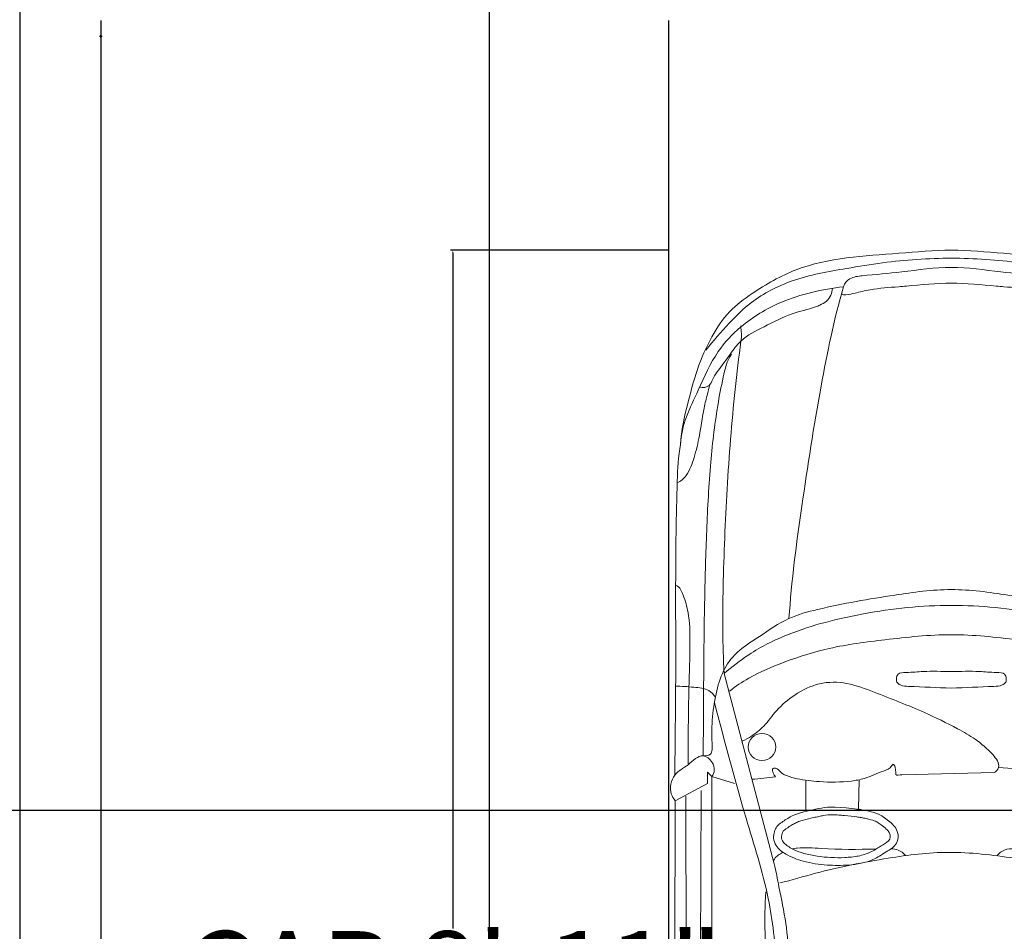
# Model space of a CAD drawing. Units: inches. Extents: x 3398 to 3816, y 15195 to 15771.
# Tile 3 of 10: x 3474 to 3547, y 15306 to 15374. Entities that reach past the tile are written whole.
import ezdxf

# ---------------------------------------------------------------- set-up
doc = ezdxf.new("R2010")
doc.units = ezdxf.units.IN
doc.header["$MEASUREMENT"] = 0
doc.layers.add('A-ANNO-DIMS', color=2, linetype='Continuous', lineweight=18)
doc.layers.add('C-PKNG-VEHI', color=8, linetype='Continuous', lineweight=13)
doc.styles.get("Standard").update_dxf_attribs({"font": 'arial.ttf'})
doc.dimstyles.get("Standard").update_dxf_attribs({"dimtxt": 6, "dimasz": 0.18, "dimexe": 0.18, "dimexo": 0.0625, "dimgap": 0.09, "dimtad": 0, "dimtih": 1, "dimtoh": 1, "dimdec": 1, "dimzin": 0, "dimdsep": 46, "dimlunit": 3, "dimtxsty": 'Standard', "dimcen": 0.09, "dimadec": 0, "dimazin": 0, "dimtfac": 1, "dimtdec": 1, "dimtofl": 0, "dimtmove": 0, "dimatfit": 3, "dimfxl": 1, "dimtolj": 1, "dimtzin": 0, "dimarcsym": 0})

# ---------------------------------------------------------------- blocks, each defined once
blk = doc.blocks.new('A$C242571DA')
for p, q in [((1659.9, 1632), (1714.3, 1732.5)), ((1714.3, 1732.5), (3817.1, 1739.9)), ((1699.9, 1699.4), (2984.7, 1695.8)), ((1681.8, 1651.6), (2695.2, 1655.3)), ((1638.3, 1618.5), (1625.1, 1632)), ((1625.1, 1632), (1659.9, 1632)), ((1638.3, 1618.5), (2503.3, 1618.5)), ((1659.9, 1548.1), (1638.3, 1618.5)), ((2503.3, 1618.5), (2861.6, 1607.5)), ((1317.4, 1579.7), (1909.8, 1424.9)), ((3007.2, 1526.5), (2808.1, 1525.2)), ((1644, 1489.1), (1610.4, 1020.2)), ((2311.9, 1454.3), (2500.6, 1456.9)), ((3474.6, 1401.1), (3474.6, 843)), ((4315.2, 1398), (4377.3, 1370.5)), ((1626.1, 1006.5), (1632.8, 719.7)), ((3474.6, 345.6), (3474.6, 903.8)), ((1740.2, 584.9), (1649.3, 586.9)), ((1746.1, 420.6), (1649.3, 420.6)), ((4315.2, 348.7), (4377.3, 376.3)), ((1317.4, 167), (1909.8, 321.9)), ((2311.9, 292.5), (2500.6, 289.8)), ((3007.2, 220.3), (2808.1, 221.6)), ((1659.9, 198.7), (1638.3, 128.2)), ((1638.3, 128.2), (1625.1, 114.7)), ((1638.3, 128.2), (2503.3, 128.2)), ((2503.3, 128.2), (2861.6, 139.2)), ((1625.1, 114.7), (1659.9, 114.7)), ((1659.9, 114.7), (1714.3, 14.2)), ((1681.8, 95.1), (2695.2, 91.4)), ((1699.9, 47.3), (2984.7, 51)), ((1714.3, 14.2), (3817.1, 6.9))]:
    blk.add_line(p, q)
for centre in [(1546.4, 1462.5), (1546.4, 284.2)]:
    blk.add_ellipse(centre, major_axis=(0, 42.9), ratio=0.983266, start_param=4.712389, end_param=10.995574)
for points, knots in [([(1714.3, 1732.5), (1707.7, 1737.6), (1683.3, 1753), (1628.7, 1741.2), (1605.6, 1691.5), (1561.7, 1652.4), (1594.1, 1610.3), (1627.9, 1608.3), (1638.3, 1618.5)], [0, 0, 0, 0, 0.024864, 0.0846267, 0.1362471, 0.1900683, 0.2245199, 0.2681841, 0.2681841, 0.2681841, 0.2681841]), ([(722.7, 1726.6), (720.8, 1714.9), (694.5, 1689.9), (643, 1671.8), (573.6, 1655.4), (508.5, 1647), (455.2, 1634.7), (428.7, 1627.3), (416.9, 1624.1)], [0, 0, 0, 0, 0.034703, 0.0959761, 0.1659336, 0.2471559, 0.2929944, 0.3295918, 0.3295918, 0.3295918, 0.3295918]), ([(604.6, 1715.7), (642.1, 1723.4), (788.5, 1729.2), (1039.3, 1732.2), (1344.5, 1729.9), (1542, 1733.1), (1633.8, 1733.7)], [0, 0, 0, 0, 0.114897, 0.437061, 0.754269, 1.029686, 1.029686, 1.029686, 1.029686]), ([(1043.6, 1729.2), (1048.6, 1717.9), (1080.9, 1704.2), (1138.6, 1687.6), (1237.7, 1685.6), (1394.7, 1691.3), (1521.7, 1692.4), (1601.5, 1692.7)], [0, 0, 0, 0, 0.0364992, 0.0923739, 0.1867837, 0.3273982, 0.5667068, 0.5667068, 0.5667068, 0.5667068]), ([(1356.8, 1732.2), (1357.1, 1712.8), (1360, 1678.8), (1363.9, 1630.5), (1383.3, 1613.5), (1391, 1607.2)], [0, 0, 0, 0, 1.462159, 2.651105, 3.386321, 3.386321, 3.386321, 3.386321]), ([(2414.7, 1735), (2424.9, 1723.3), (2447.2, 1698.8), (2461.2, 1657.6), (2468.1, 1629), (2468, 1616.1)], [1.808086, 1.808086, 1.808086, 1.808086, 2.918874, 4.131288, 5.10151, 5.10151, 5.10151, 5.10151]), ([(3356.5, 1739.4), (3354.9, 1719.2), (3360.8, 1678.2), (3324, 1631.5), (3255.4, 1544.3), (3187.1, 1476.2), (3125.2, 1432.2)], [0, 0, 0, 0, 0.0597371, 0.1139981, 0.1672498, 0.3938869, 0.3938869, 0.3938869, 0.3938869]), ([(3745.3, 1736.8), (3748.5, 1730.1), (3764.2, 1717.1), (3811.5, 1698.6), (3894.7, 1686.7), (4002.9, 1663.2), (4107.9, 1648.7), (4195.8, 1638.3), (4258.6, 1603.2), (4302.1, 1549.7), (4339.9, 1483.8), (4365.2, 1407.6), (4389.6, 1324.4), (4397.9, 1266.9), (4401.8, 1235.2)], [0, 0, 0, 0, 0.0219205, 0.0572122, 0.1522539, 0.2718866, 0.3894011, 0.4710097, 0.5346344, 0.5986698, 0.6733118, 0.758696, 0.8351341, 0.9293726, 0.9293726, 0.9293726, 0.9293726]), ([(3817.1, 1739.9), (3833.2, 1729.7), (3882.9, 1718.2), (3973.3, 1695.2), (4085.1, 1680.5), (4193.8, 1662.8), (4280.6, 1644.3), (4343.9, 1598.1), (4390, 1540.3), (4427.4, 1448.7), (4457.8, 1336.6), (4475.7, 1233.4), (4478.4, 1175.1), (4479.3, 1161.6)], [0, 0, 0, 0, 0.056668, 0.14946, 0.28161, 0.392935, 0.481686, 0.542967, 0.622845, 0.69797, 0.833643, 0.965665, 1.00577, 1.00577, 1.00577, 1.00577]), ([(0, 873.4), (0, 927.8), (15.6, 1088.6), (25.5, 1309.8), (120.7, 1476.4), (189.2, 1569), (273.5, 1623.1), (369.9, 1666.3), (483, 1694.7), (561.3, 1714.9), (604.6, 1715.7)], [0, 0, 0, 0, 0.16039, 0.479033, 0.632967, 0.722015, 0.817474, 0.927562, 1.03733, 1.167094, 1.167094, 1.167094, 1.167094]), ([(604.6, 1715.7), (545.5, 1714.5), (448.5, 1664.6), (320.8, 1610.6), (225.4, 1521.2), (147.3, 1390.5), (121.7, 1275.2), (113.6, 1208.7)], [0, 0, 0, 0, 0.1772572, 0.3124951, 0.4151678, 0.5597243, 0.7575412, 0.7575412, 0.7575412, 0.7575412]), ([(2984.7, 1695.8), (3051, 1695.6), (3172.1, 1691.3), (3367.4, 1677.6), (3575.2, 1664.3), (3788.2, 1643.6), (3968, 1628.1), (4103.8, 1616.8), (4203.6, 1578.1), (4271.8, 1519.5), (4300.6, 1452.1), (4341.7, 1305.3), (4361.8, 1111.2), (4367.5, 936.8), (4367.5, 873.4)], [0, 0, 0, 0, 0.198873, 0.363323, 0.587433, 0.823543, 1.004622, 1.129816, 1.230113, 1.320655, 1.388577, 1.443334, 1.771447, 1.958652, 1.958652, 1.958652, 1.958652]), ([(426.8, 1656.7), (428.5, 1646.6), (426.9, 1625), (399.8, 1616.6), (368.1, 1593.9), (328, 1564.6), (271.6, 1523.9), (237, 1451.9), (196.2, 1376.7), (183.8, 1314.9), (170, 1279.6), (157.2, 1254.2), (133.3, 1244.4), (118.6, 1242.9)], [0, 0, 0, 0, 0.0304541, 0.0502818, 0.0786089, 0.1479133, 0.1986294, 0.2831705, 0.3780326, 0.4523267, 0.4667809, 0.4902599, 0.5347198, 0.5347198, 0.5347198, 0.5347198]), ([(2695.2, 1655.3), (2829.9, 1655.3), (3041.2, 1651.4), (3351.3, 1630.7), (3527.5, 1623.2), (3626.6, 1612)], [0, 0, 0, 0, 0.4042759, 0.6333827, 0.9326252, 0.9326252, 0.9326252, 0.9326252]), ([(310.7, 1637.3), (282.5, 1613.7), (230.1, 1569.9), (148.7, 1486.2), (84.8, 1361.3), (60, 1219), (32.6, 1054.3), (25.1, 944.9), (25.1, 873.4)], [0, 0, 0, 0, 0.1095129, 0.2035347, 0.3452507, 0.5161382, 0.6275464, 0.8383798, 0.8383798, 0.8383798, 0.8383798]), ([(323.7, 1557.5), (344.8, 1571.9), (400.4, 1585.1), (516, 1606.8), (680.3, 1625.8), (885.4, 1635.7), (1116.8, 1642.2), (1346.1, 1644.2), (1504.7, 1644.7), (1574, 1645.7)], [0, 0, 0, 0, 0.076148, 0.165903, 0.355672, 0.569871, 0.782325, 1.050047, 1.257936, 1.257936, 1.257936, 1.257936]), ([(1574, 1645.7), (1572.9, 1638), (1574.1, 1622), (1559.9, 1618.7), (1555.2, 1617.8)], [0, 0, 0, 0, 0.02274132, 0.03717479, 0.03717479, 0.03717479, 0.03717479]), ([(1555.2, 1617.8), (1527.7, 1617.8), (1472.5, 1620.4), (1392.7, 1608.8), (1318.5, 1591), (1249.4, 1545.5), (1201.4, 1466.7), (1142.8, 1385.7), (1104.8, 1240.4), (1076, 1072.3), (1056.4, 932.4), (1056.4, 873.4)], [0, 0, 0, 0, 0.082256, 0.165174, 0.241383, 0.30939, 0.405348, 0.511507, 0.603349, 0.843635, 1.017671, 1.017671, 1.017671, 1.017671]), ([(3535.9, 1563.1), (3520.1, 1550.9), (3484.4, 1526.1), (3408.2, 1510.9), (3323.4, 1473.1), (3207.9, 1445), (3072.6, 1422.2), (2866.9, 1404.6), (2626.4, 1412.9), (2396.7, 1410.8), (2200.9, 1416.9), (2001.3, 1438.2), (1732.1, 1525.9), (1527.9, 1578.9), (1407.5, 1610.7)], [0, 0, 0, 0, 0.05975, 0.126928, 0.230034, 0.336675, 0.482225, 0.641324, 0.954906, 1.203173, 1.330375, 1.542773, 1.802261, 2.175545, 2.175545, 2.175545, 2.175545]), ([(2424, 1618.7), (2441.5, 1589.9), (2464.2, 1518.9), (2495.4, 1450.9), (2501.6, 1411.3)], [0, 0, 0, 0, 0.1000351, 0.2184418, 0.2184418, 0.2184418, 0.2184418]), ([(2507.7, 1618.4), (2521, 1587.7), (2536.6, 1527.1), (2559.6, 1458.5), (2563.3, 1420.6), (2563.8, 1411.4)], [0, 0, 0, 0, 2.528586, 4.711885, 5.408215, 5.408215, 5.408215, 5.408215]), ([(2861.6, 1607.5), (2921.1, 1607.3), (3047.2, 1600.8), (3191.4, 1602), (3356.6, 1584.1), (3498.3, 1570.6), (3623.2, 1549.4), (3664.1, 1533.3)], [0, 0, 0, 0, 0.1783018, 0.3787173, 0.431954, 0.6762374, 0.8077184, 0.8077184, 0.8077184, 0.8077184]), ([(3248.1, 1545.2), (3226.9, 1550.4), (3176.1, 1562.1), (3113.7, 1592.9), (3052.6, 1605.3), (3010.4, 1578.8), (3010.3, 1545.3), (3010.3, 1515.9), (3033.7, 1500.1), (3052.6, 1465.2), (3078.9, 1443.5), (3084, 1424.4)], [0, 0, 0, 0, 0.0655106, 0.1550445, 0.2094604, 0.2438604, 0.287164, 0.3001388, 0.3275984, 0.3616951, 0.4200969, 0.4200969, 0.4200969, 0.4200969]), ([(3626.6, 1612), (3702.5, 1609.1), (3826.2, 1596.8), (3991.4, 1583.2), (4111.7, 1562.4), (4212.2, 1522.7), (4290.4, 1488), (4300.7, 1447.5)], [0, 0, 0, 0, 0.2277977, 0.3719478, 0.4996814, 0.5863441, 0.709615, 0.709615, 0.709615, 0.709615]), ([(1317.4, 1579.7), (1227.8, 1586.1), (1036, 1584.8), (741.2, 1572.5), (486.1, 1553.3), (333.3, 1534.3), (283.3, 1528.5)], [0, 0, 0, 0, 0.269375, 0.574535, 0.885339, 1.036319, 1.036319, 1.036319, 1.036319]), ([(1317.4, 1579.7), (1296.6, 1555.5), (1247.9, 1494.4), (1177.6, 1350.5), (1124.2, 1137.4), (1105.5, 964.9), (1105.5, 873.4)], [0, 0, 0, 0, 0.0947759, 0.2311242, 0.4700259, 0.7400315, 0.7400315, 0.7400315, 0.7400315]), ([(1372.8, 1563.1), (1357.2, 1545), (1321.6, 1490.1), (1277, 1385.7), (1232.8, 1244.2), (1211.1, 1069.4), (1196.8, 942.4), (1196.8, 873.4)], [0, 0, 0, 0, 0.0708922, 0.1925846, 0.3348457, 0.5072814, 0.7109928, 0.7109928, 0.7109928, 0.7109928]), ([(3319, 1587.1), (3303.3, 1568.1), (3256.9, 1516.7), (3206.7, 1467.3), (3171.4, 1439.5)], [0, 0, 0, 0, 1.868162, 5.271297, 5.271297, 5.271297, 5.271297]), ([(3275.5, 1532.8), (3287.5, 1528.3), (3299.8, 1504.9), (3308.4, 1482.5), (3311.7, 1472.6)], [0, 0, 0, 0, 0.983949, 1.771691, 1.771691, 1.771691, 1.771691]), ([(3372.2, 1495.3), (3354.4, 1496.8), (3316, 1494.7), (3291.6, 1525.8), (3275.5, 1532.8)], [0, 0, 0, 0, 0.0535488, 0.1060573, 0.1060573, 0.1060573, 0.1060573]), ([(3664.1, 1533.3), (3687, 1526), (3734.8, 1502.3), (3816.7, 1444.8), (3884.1, 1342.9), (3925.1, 1239.9), (3937.3, 1177), (3940.4, 1157.6)], [0, 0, 0, 0, 0.0720749, 0.1581284, 0.2958089, 0.4262456, 0.4842292, 0.4842292, 0.4842292, 0.4842292]), ([(2808.1, 1525.2), (2791.9, 1525.1), (2751.9, 1519.7), (2710.6, 1472.6), (2690, 1431.1), (2690.5, 1409.6)], [0, 0, 0, 0, 0.0486628, 0.1144515, 0.1777721, 0.1777721, 0.1777721, 0.1777721]), ([(1909.8, 1424.9), (1933.5, 1418.7), (1995.6, 1407.6), (2094.4, 1385.8), (2211.8, 1377.1), (2419, 1366.9), (2704.7, 1366.5), (3032.7, 1354.2), (3316.2, 1371), (3558.7, 1415.9), (3789.1, 1461.7), (4028.9, 1452.9), (4196.2, 1455.2), (4292.7, 1447.9), (4300.7, 1447.5)], [0, 0, 0, 0, 0.073325, 0.188896, 0.303039, 0.425821, 0.811242, 1.159737, 1.41058, 1.660623, 1.899627, 2.11145, 2.377727, 2.401703, 2.401703, 2.401703, 2.401703]), ([(1997.2, 1450.5), (2039.7, 1454.5), (2126.7, 1451.9), (2219.8, 1454.5), (2287.1, 1456.9), (2305.7, 1434.4), (2313.2, 1419.9), (2315.8, 1413.5)], [0, 0, 0, 0, 3.267856, 6.568708, 7.399663, 8.099385, 8.621705, 8.621705, 8.621705, 8.621705]), ([(1898.5, 1426.2), (1889, 1420.6), (1871, 1397.2), (1856.4, 1345.2), (1867.7, 1233.5), (1864.3, 1132.3), (1863, 1038.5), (1876.9, 1022.3), (1884.5, 1015.7)], [0, 0, 0, 0, 0.842998, 2.122875, 3.997599, 9.174838, 10.012722, 10.751336, 10.751336, 10.751336, 10.751336]), ([(1969.6, 1407.3), (1960.5, 1369.8), (1927, 1259.1), (1890.9, 1078.4), (1874.3, 933), (1874.3, 864.4)], [0, 0, 0, 0, 0.1139079, 0.3411539, 0.543502, 0.543502, 0.543502, 0.543502]), ([(113.6, 1208.7), (215.2, 1238.6), (443.2, 1284.9), (788, 1338.7), (1029.5, 1370.7), (1146.4, 1378.6)], [0, 0, 0, 0, 0.317374, 0.69576, 1.04714, 1.04714, 1.04714, 1.04714]), ([(3231.5, 1368.3), (3240.8, 1356.2), (3253.1, 1315.7), (3271.9, 1240.7), (3297.9, 1127.9), (3310.5, 974.6), (3311.2, 858.3), (3311.6, 794.4)], [0, 0, 0, 0, 0.0451009, 0.1211996, 0.2308505, 0.385263, 0.5739042, 0.5739042, 0.5739042, 0.5739042]), ([(3294.8, 1174.5), (3294.8, 1207.4), (3299.6, 1249.5), (3298.3, 1303.9), (3326.3, 1329), (3363.9, 1320.7), (3399.3, 1329.3), (3422.1, 1315.7), (3430.7, 1297.9), (3438.7, 1234.2), (3439.6, 1174.4), (3434.7, 1112.2), (3418.9, 1102), (3395.9, 1098.6), (3362.6, 1100.9), (3331.1, 1096.6), (3298.8, 1107.6), (3297.3, 1140.3), (3294.8, 1160.9), (3294.8, 1174.5)], [0, 0, 0, 0, 0.0969044, 0.1295913, 0.1506192, 0.1985921, 0.2360698, 0.2557908, 0.2719711, 0.2929882, 0.44406, 0.4519132, 0.4720918, 0.4918599, 0.5228758, 0.5707096, 0.5892096, 0.6145759, 0.654681, 0.654681, 0.654681, 0.654681]), ([(4401.8, 1235.2), (4411.9, 1185.3), (4421.6, 1065.8), (4424.1, 946.5), (4424.1, 878)], [0, 0, 0, 0, 0.1502861, 0.3522699, 0.3522699, 0.3522699, 0.3522699]), ([(113.6, 1208.7), (103.3, 1207), (83.6, 1187.6), (76.5, 1122.2), (68.2, 1017.3), (53.4, 925), (53.4, 873.4)], [0, 0, 0, 0, 0.0314754, 0.0702057, 0.1915753, 0.3439346, 0.3439346, 0.3439346, 0.3439346]), ([(135.5, 1213.1), (139.1, 1211.8), (138.4, 1193.3), (132.6, 1168.3), (118.8, 1111.9), (115.6, 1058.9), (109, 974.6), (102.4, 920.1), (102.4, 873.4)], [0, 0, 0, 0, 0.0114788, 0.0403472, 0.0875838, 0.1755608, 0.1991501, 0.3369659, 0.3369659, 0.3369659, 0.3369659]), ([(3940.4, 1157.6), (3949.9, 1111), (3964.3, 1016.4), (3960.5, 921), (3959.8, 873.4)], [0, 0, 0, 0, 0.140379, 0.2808468, 0.2808468, 0.2808468, 0.2808468]), ([(3339.2, 1099), (3339.1, 1094.8), (3336.4, 1010.6), (3333.2, 926.3), (3330, 846.2)], [11.235438, 11.235438, 11.235438, 11.235438, 11.552536, 17.586883, 17.586883, 17.586883, 17.586883]), ([(1311.3, 873.4), (1311.2, 902.4), (1309.2, 950.9), (1315, 1002.2), (1314.2, 1039.4), (1332.1, 1044.9), (1345.7, 1044.2), (1356.8, 1028.5), (1359.2, 970.2), (1361.5, 917.6), (1362.9, 873.4)], [0, 0, 0, 0, 0.0857277, 0.1381048, 0.1641986, 0.1769751, 0.1890325, 0.2028129, 0.2286049, 0.3592554, 0.3592554, 0.3592554, 0.3592554]), ([(1626.1, 1006.5), (1623.5, 1013), (1603.1, 1029.4), (1559.1, 995), (1523, 951.9), (1480.3, 878.3), (1430.5, 774.3), (1385.5, 658.5), (1343.7, 551.3), (1343, 461.7), (1380.3, 386.9), (1428.2, 329.9), (1480.1, 294.6), (1509.8, 257.4), (1524.8, 232.6), (1528, 222.1)], [0, 0, 0, 0, 0.527288, 1.647451, 3.487558, 5.099073, 7.968657, 12.238313, 14.475187, 16.613757, 18.744202, 20.639343, 22.223389, 23.452731, 24.286529, 24.286529, 24.286529, 24.286529]), ([(3231.5, 378.5), (3240.8, 390.5), (3253.1, 431), (3271.9, 506.1), (3297.9, 618.9), (3310.5, 772.1), (3311.2, 888.4), (3311.6, 952.4)], [0, 0, 0, 0, 0.0451009, 0.1211996, 0.2308505, 0.385263, 0.5739042, 0.5739042, 0.5739042, 0.5739042]), ([(3339.2, 647.8), (3339.1, 652), (3336.4, 736.2), (3333.2, 820.5), (3330, 900.6)], [11.235438, 11.235438, 11.235438, 11.235438, 11.552536, 17.586883, 17.586883, 17.586883, 17.586883]), ([(0, 873.4), (0, 819), (15.6, 658.1), (25.5, 437), (120.7, 270.3), (189.2, 177.8), (273.5, 123.7), (369.9, 80.4), (483, 52), (561.3, 31.9), (604.6, 31)], [0, 0, 0, 0, 0.16039, 0.479033, 0.632967, 0.722015, 0.817474, 0.927562, 1.03733, 1.167094, 1.167094, 1.167094, 1.167094]), ([(310.7, 109.5), (282.5, 133.1), (230.1, 176.9), (148.7, 260.5), (84.8, 385.5), (60, 527.8), (32.6, 692.4), (25.1, 801.9), (25.1, 873.4)], [0, 0, 0, 0, 0.1095129, 0.2035347, 0.3452507, 0.5161382, 0.6275464, 0.8383798, 0.8383798, 0.8383798, 0.8383798]), ([(113.6, 538.1), (103.3, 539.8), (83.6, 559.2), (76.5, 624.5), (68.2, 729.4), (53.4, 821.7), (53.4, 873.4)], [0, 0, 0, 0, 0.0314754, 0.0702057, 0.1915753, 0.3439346, 0.3439346, 0.3439346, 0.3439346]), ([(135.5, 533.6), (139.1, 534.9), (138.4, 553.4), (132.6, 578.4), (118.8, 634.9), (115.6, 687.8), (109, 772.2), (102.4, 826.7), (102.4, 873.4)], [0, 0, 0, 0, 0.0114788, 0.0403472, 0.0875838, 0.1755608, 0.1991501, 0.3369659, 0.3369659, 0.3369659, 0.3369659]), ([(1555.2, 129), (1527.7, 129), (1472.5, 126.3), (1392.7, 138), (1318.5, 155.7), (1249.4, 201.3), (1201.4, 280.1), (1142.8, 361.1), (1104.8, 506.4), (1076, 674.5), (1056.4, 814.4), (1056.4, 873.4)], [0, 0, 0, 0, 0.082256, 0.165174, 0.241383, 0.30939, 0.405348, 0.511507, 0.603349, 0.843635, 1.017671, 1.017671, 1.017671, 1.017671]), ([(1317.4, 167), (1296.6, 191.2), (1247.9, 252.4), (1177.6, 396.3), (1124.2, 609.4), (1105.5, 781.8), (1105.5, 873.4)], [0, 0, 0, 0, 0.0947759, 0.2311242, 0.4700259, 0.7400315, 0.7400315, 0.7400315, 0.7400315]), ([(1372.8, 183.6), (1357.2, 201.8), (1321.6, 256.7), (1277, 361), (1232.8, 502.6), (1211.1, 677.3), (1196.8, 804.3), (1196.8, 873.4)], [0, 0, 0, 0, 0.0708922, 0.1925846, 0.3348457, 0.5072814, 0.7109928, 0.7109928, 0.7109928, 0.7109928]), ([(1311.3, 873.4), (1311.2, 844.3), (1309.2, 795.8), (1315, 744.6), (1314.2, 707.4), (1332.1, 701.9), (1345.7, 702.6), (1356.8, 718.2), (1359.2, 776.6), (1361.5, 829.1), (1362.9, 873.4)], [0, 0, 0, 0, 0.0857277, 0.1381048, 0.1641986, 0.1769751, 0.1890325, 0.2028129, 0.2286049, 0.3592554, 0.3592554, 0.3592554, 0.3592554]), ([(1969.6, 339.5), (1960.5, 377), (1926.9, 487.6), (1892.9, 662.7), (1874.3, 801.8), (1874.3, 864.4)], [0, 0, 0, 0, 0.1139079, 0.3411539, 0.5260188, 0.5260188, 0.5260188, 0.5260188]), ([(2984.7, 51), (3051, 51.1), (3172.1, 55.5), (3367.4, 69.2), (3575.2, 82.5), (3788.2, 103.1), (3968, 118.7), (4103.8, 130), (4203.6, 168.6), (4271.8, 227.3), (4300.6, 294.7), (4341.7, 441.5), (4361.8, 635.5), (4367.5, 809.9), (4367.5, 873.4)], [0, 0, 0, 0, 0.198873, 0.363323, 0.587433, 0.823543, 1.004622, 1.129816, 1.230113, 1.320655, 1.388577, 1.443334, 1.771447, 1.958652, 1.958652, 1.958652, 1.958652]), ([(3940.4, 589.1), (3949.9, 635.7), (3964.3, 730.4), (3960.5, 825.8), (3959.8, 873.4)], [0, 0, 0, 0, 0.140379, 0.2808468, 0.2808468, 0.2808468, 0.2808468]), ([(4401.8, 511.5), (4411.9, 561.5), (4421.6, 681), (4424.1, 800.3), (4424.1, 868.8)], [0, 0, 0, 0, 0.1502861, 0.3522699, 0.3522699, 0.3522699, 0.3522699]), ([(1639.2, 326.1), (1635.3, 323.6), (1629, 318.4), (1613.1, 314.9), (1612, 324.2), (1613.2, 330.4), (1619, 337.5), (1629, 345.7), (1637.9, 366.1), (1649, 404.8), (1656.3, 472.9), (1656.2, 543.1), (1644.6, 610.9), (1623, 651.2), (1615, 684.3), (1598.5, 691.2), (1604, 696.6), (1610.3, 699.7), (1618.8, 698.9), (1625.9, 701.3), (1638.1, 698.6), (1633, 713.4), (1632.8, 719.7)], [0, 0, 0, 0, 0.0138597, 0.0278304, 0.0329137, 0.0379971, 0.0465756, 0.0592704, 0.0762214, 0.1105991, 0.1789801, 0.2766959, 0.3173629, 0.3800771, 0.4110544, 0.4160421, 0.4210284, 0.4277212, 0.4387433, 0.4448131, 0.4508005, 0.4694463, 0.4694463, 0.4694463, 0.4694463]), ([(1740.2, 584.9), (1737.8, 571.7), (1749.5, 644.3), (1766.4, 664.5), (1792.2, 700.2), (1821.5, 709.7), (1853.1, 703.9), (1874, 668.4), (1904.5, 622.6), (1915.6, 557.2), (1915.1, 484.2), (1905.7, 417.6), (1884.9, 362.8), (1859.3, 329.1), (1831.3, 318.1), (1810.8, 322.7), (1792.2, 329.3), (1777.9, 350.3), (1753, 385.9), (1737.9, 465.8), (1728.8, 497.3), (1742.4, 597.6), (1740.2, 584.9)], [0, 0, 0, 0, 0.03969, 0.089634, 0.13125, 0.1542862, 0.1797268, 0.2207266, 0.2680991, 0.3447665, 0.4095645, 0.4843001, 0.541515, 0.5817687, 0.6060665, 0.6262474, 0.6436722, 0.6634686, 0.6988791, 0.7758465, 0.8696394, 0.907731, 0.907731, 0.907731, 0.907731]), ([(1863.4, 685.6), (1863.6, 693.5), (1865.3, 711), (1876.9, 724.5), (1884.5, 731)], [9.436432, 9.436432, 9.436432, 9.436432, 10.012722, 10.751336, 10.751336, 10.751336, 10.751336]), ([(1764.9, 587), (1765.6, 590.8), (1766.4, 595.5), (1768.5, 605.7), (1769.7, 611.3), (1773.4, 626.6), (1775.6, 633), (1779.7, 642.1), (1781.6, 644.9), (1785.7, 650.6), (1787.1, 652.5), (1793, 660.3), (1797.4, 666.2), (1804.2, 673.7), (1806.8, 676.1), (1811.1, 679.4), (1812.9, 680.5), (1816.8, 682.1), (1818.8, 682.7), (1824.4, 683.5), (1828.3, 683.2), (1832.5, 682), (1833.6, 681.5), (1836, 680.2), (1837.9, 678.7), (1842.4, 673.7), (1844.9, 670.1), (1850.3, 661.7), (1853.4, 656.6), (1859.3, 647.3), (1862.1, 642.8), (1868.3, 632.6), (1871.4, 626.9), (1876.7, 615.7), (1878.9, 609.8), (1882.8, 597.4), (1884.4, 590.8), (1888.3, 570.5), (1889.7, 556.1), (1891.2, 527.4), (1891.1, 513.1), (1888.9, 470), (1885.1, 441.2), (1874.3, 404), (1870.6, 393.8), (1863.5, 378.7), (1860.6, 373.4), (1854.4, 363.6), (1851.2, 359.2), (1845, 352.6), (1842, 350.2), (1835.8, 346.4), (1832.6, 345.3), (1828.8, 344.6), (1827.9, 344.6), (1824.6, 344.9), (1822.6, 345.2), (1817.8, 346.4), (1814.9, 347.3), (1810.9, 348.7), (1809.4, 349.4), (1808.3, 350.1), (1808.1, 350.2), (1807.3, 351), (1806.7, 351.6), (1804.7, 354), (1803.1, 356.2), (1799.6, 361.3), (1798, 363.7), (1794.9, 368.2), (1793.4, 370.4), (1789.2, 376.9), (1786.7, 381), (1782.4, 389.3), (1780.5, 393.6), (1776.9, 403), (1775.2, 408), (1770.7, 423.5), (1768.3, 434.2), (1764.9, 450.5), (1763.6, 456.4), (1761.4, 466.8), (1760.4, 471.4), (1758.1, 484.4), (1757.3, 492.6), (1757.5, 510.7), (1757.8, 516.5), (1758.6, 528.4), (1759.1, 534.3), (1761.1, 553.9), (1763.1, 570.6), (1764.4, 581.5), (1764.6, 583), (1764.7, 585), (1764.8, 585.5), (1764.8, 586.5), (1764.8, 586.7), (1764.9, 587)], [0.497033, 0.497033, 0.497033, 0.497033, 0.723444, 0.723444, 0.974636, 0.974636, 1.50964, 1.50964, 2.044645, 2.044645, 2.271061, 2.271061, 2.862376, 2.862376, 3.217654, 3.217654, 3.537253, 3.537253, 3.856852, 3.856852, 4.368613, 4.368613, 4.584627, 4.584627, 4.99269, 4.99269, 5.400753, 5.400753, 5.808816, 5.808816, 6.216879, 6.216879, 6.778716, 6.778716, 7.350371, 7.350371, 7.922025, 7.922025, 9.065335, 9.065335, 10.208644, 10.208644, 12.495263, 12.495263, 13.409896, 13.409896, 13.929088, 13.929088, 14.44828, 14.44828, 14.909885, 14.909885, 15.371489, 15.371489, 15.62524, 15.62524, 15.87899, 15.87899, 16.120875, 16.120875, 16.36276, 16.36276, 16.51635, 16.51635, 16.669941, 16.669941, 16.921521, 16.921521, 17.136676, 17.136676, 17.351831, 17.351831, 17.782142, 17.782142, 18.204974, 18.204974, 18.627807, 18.627807, 19.473473, 19.473473, 19.978923, 19.978923, 20.484372, 20.484372, 21.475119, 21.475119, 21.859144, 21.859144, 22.162884, 22.162884, 22.770362, 22.770362, 22.900493, 22.900493, 22.951221, 22.951221, 22.964298, 22.964298, 22.964298, 22.964298]), ([(3294.8, 572.3), (3294.8, 539.4), (3299.6, 497.2), (3298.3, 442.9), (3326.3, 417.8), (3363.9, 426), (3399.3, 417.5), (3422.1, 431), (3430.7, 448.9), (3438.7, 512.5), (3439.6, 572.4), (3434.7, 634.6), (3418.9, 644.7), (3395.9, 648.2), (3362.6, 645.9), (3331.1, 650.1), (3298.8, 639.2), (3297.3, 606.5), (3294.8, 585.9), (3294.8, 572.3)], [0, 0, 0, 0, 0.0969044, 0.1295913, 0.1506192, 0.1985921, 0.2360698, 0.2557908, 0.2719711, 0.2929882, 0.44406, 0.4519132, 0.4720918, 0.4918599, 0.5228758, 0.5707096, 0.5892096, 0.6145759, 0.654681, 0.654681, 0.654681, 0.654681]), ([(1863.7, 379.4), (1862.6, 384.2), (1857.6, 413.7), (1866.5, 501.6), (1865.2, 581.4), (1864.1, 639.5)], [1.749253, 1.749253, 1.749253, 1.749253, 2.122875, 3.997599, 8.307432, 8.307432, 8.307432, 8.307432]), ([(3664.1, 213.5), (3687, 220.8), (3734.8, 244.4), (3816.7, 302), (3884.1, 403.8), (3925.1, 506.9), (3937.3, 569.7), (3940.4, 589.1)], [0, 0, 0, 0, 0.0720749, 0.1581284, 0.2958089, 0.4262456, 0.4842292, 0.4842292, 0.4842292, 0.4842292]), ([(3817.1, 6.9), (3833.2, 17), (3882.9, 28.6), (3973.3, 51.5), (4085.1, 66.3), (4193.8, 84), (4280.6, 102.4), (4343.9, 148.6), (4390, 206.4), (4427.4, 298), (4457.8, 410.1), (4475.7, 513.3), (4478.4, 571.6), (4479.3, 585.2)], [0, 0, 0, 0, 0.056668, 0.14946, 0.28161, 0.392935, 0.481686, 0.542967, 0.622845, 0.69797, 0.833643, 0.965665, 1.00577, 1.00577, 1.00577, 1.00577]), ([(604.6, 31), (545.5, 32.3), (448.5, 82.2), (320.8, 136.1), (225.4, 225.5), (147.3, 356.2), (121.7, 471.5), (113.6, 538.1)], [0, 0, 0, 0, 0.1772572, 0.3124951, 0.4151678, 0.5597243, 0.7575412, 0.7575412, 0.7575412, 0.7575412]), ([(113.6, 538.1), (215.2, 508.2), (443.2, 461.9), (788, 408.1), (1029.5, 376), (1146.4, 368.2)], [0, 0, 0, 0, 0.317374, 0.69576, 1.04714, 1.04714, 1.04714, 1.04714]), ([(426.8, 90), (428.5, 100.2), (426.9, 121.8), (399.8, 130.1), (368.1, 152.8), (328, 182.2), (271.6, 222.8), (237, 294.9), (196.2, 370.1), (183.8, 431.9), (170, 467.2), (157.2, 492.6), (133.3, 502.4), (118.6, 503.9)], [0, 0, 0, 0, 0.0304541, 0.0502818, 0.0786089, 0.1479133, 0.1986294, 0.2831705, 0.3780326, 0.4523267, 0.4667809, 0.4902599, 0.5347198, 0.5347198, 0.5347198, 0.5347198]), ([(3745.3, 10), (3748.5, 16.7), (3764.2, 29.7), (3811.5, 48.1), (3894.7, 60.1), (4002.9, 83.6), (4107.9, 98), (4195.8, 108.4), (4258.6, 143.5), (4302.1, 197), (4339.9, 262.9), (4365.2, 339.2), (4389.6, 422.4), (4397.9, 479.8), (4401.8, 511.5)], [0, 0, 0, 0, 0.0219205, 0.0572122, 0.1522539, 0.2718866, 0.3894011, 0.4710097, 0.5346344, 0.5986698, 0.6733118, 0.758696, 0.8351341, 0.9293726, 0.9293726, 0.9293726, 0.9293726]), ([(1909.8, 321.9), (1933.5, 328.1), (1995.6, 339.2), (2094.4, 361), (2211.8, 369.6), (2419, 379.8), (2704.7, 380.3), (3032.7, 392.6), (3316.2, 375.8), (3558.7, 330.9), (3789.1, 285.1), (4028.9, 293.9), (4196.2, 291.5), (4292.7, 298.8), (4300.7, 299.2)], [0, 0, 0, 0, 0.073325, 0.188896, 0.303039, 0.425821, 0.811242, 1.159737, 1.41058, 1.660623, 1.899627, 2.11145, 2.377727, 2.401703, 2.401703, 2.401703, 2.401703]), ([(3535.9, 183.7), (3520.1, 195.9), (3484.4, 220.6), (3408.2, 235.8), (3323.4, 273.7), (3207.9, 301.8), (3072.6, 324.6), (2866.9, 342.1), (2626.4, 333.8), (2396.7, 335.9), (2200.9, 329.9), (2001.3, 308.6), (1732.1, 220.8), (1527.9, 167.8), (1407.5, 136)], [0, 0, 0, 0, 0.05975, 0.126928, 0.230034, 0.336675, 0.482225, 0.641324, 0.954906, 1.203173, 1.330375, 1.542773, 1.802261, 2.175545, 2.175545, 2.175545, 2.175545]), ([(1898.5, 320.6), (1889, 326.2), (1880.8, 336.8), (1874.8, 348.3), (1874, 349.7)], [0, 0, 0, 0, 0.8429982, 0.9626806, 0.9626806, 0.9626806, 0.9626806]), ([(2808.1, 221.6), (2791.9, 221.6), (2751.9, 227.1), (2710.6, 274.2), (2690, 315.7), (2690.5, 337.1)], [0, 0, 0, 0, 0.0486628, 0.1144515, 0.1777721, 0.1777721, 0.1777721, 0.1777721]), ([(1997.2, 296.3), (2039.7, 292.2), (2126.7, 294.9), (2219.8, 292.3), (2287.1, 289.9), (2305.7, 312.3), (2313.2, 326.9), (2315.8, 333.2)], [0, 0, 0, 0, 3.267856, 6.568708, 7.399663, 8.099385, 8.621705, 8.621705, 8.621705, 8.621705]), ([(2424, 128), (2441.5, 156.9), (2464.2, 227.8), (2495.4, 295.8), (2501.6, 335.5)], [0, 0, 0, 0, 0.1000351, 0.2184418, 0.2184418, 0.2184418, 0.2184418]), ([(2507.7, 128.3), (2521, 159.1), (2536.6, 219.7), (2559.6, 288.3), (2563.3, 326.1), (2563.8, 335.3)], [0, 0, 0, 0, 2.528586, 4.711885, 5.408215, 5.408215, 5.408215, 5.408215]), ([(3248.1, 201.6), (3226.9, 196.3), (3176.1, 184.7), (3113.7, 153.8), (3052.6, 141.4), (3010.4, 168), (3010.3, 201.5), (3010.3, 230.9), (3033.7, 246.6), (3052.6, 281.6), (3078.9, 303.2), (3084, 322.4)], [0, 0, 0, 0, 0.0655106, 0.1550445, 0.2094604, 0.2438604, 0.287164, 0.3001388, 0.3275984, 0.3616951, 0.4200969, 0.4200969, 0.4200969, 0.4200969]), ([(3356.5, 7.4), (3354.9, 27.5), (3360.8, 68.5), (3324, 115.2), (3255.4, 202.5), (3187.1, 270.5), (3125.2, 314.6)], [0, 0, 0, 0, 0.0597371, 0.1139981, 0.1672498, 0.3938869, 0.3938869, 0.3938869, 0.3938869]), ([(3319, 159.7), (3303.3, 178.6), (3256.9, 230), (3206.7, 279.5), (3171.4, 307.2)], [0, 0, 0, 0, 1.868162, 5.271297, 5.271297, 5.271297, 5.271297]), ([(3626.6, 134.7), (3702.5, 137.7), (3826.2, 149.9), (3991.4, 163.5), (4111.7, 184.4), (4212.2, 224.1), (4290.4, 258.8), (4300.7, 299.2)], [0, 0, 0, 0, 0.2277977, 0.3719478, 0.4996814, 0.5863441, 0.709615, 0.709615, 0.709615, 0.709615]), ([(3275.5, 214), (3287.5, 218.5), (3299.8, 241.9), (3308.4, 264.3), (3311.7, 274.2)], [0, 0, 0, 0, 0.983949, 1.771691, 1.771691, 1.771691, 1.771691]), ([(3372.2, 251.5), (3354.4, 249.9), (3316, 252), (3291.6, 220.9), (3275.5, 214)], [0, 0, 0, 0, 0.0535488, 0.1060573, 0.1060573, 0.1060573, 0.1060573]), ([(1317.4, 167), (1227.8, 160.7), (1036, 161.9), (741.2, 174.2), (486.1, 193.4), (333.3, 212.5), (283.3, 218.3)], [0, 0, 0, 0, 0.269375, 0.574535, 0.885339, 1.036319, 1.036319, 1.036319, 1.036319]), ([(323.7, 189.2), (344.8, 174.9), (400.4, 161.7), (516, 139.9), (680.3, 121), (885.4, 111), (1116.8, 104.5), (1346.1, 102.5), (1504.7, 102), (1574, 101.1)], [0, 0, 0, 0, 0.076148, 0.165903, 0.355672, 0.569871, 0.782325, 1.050047, 1.257936, 1.257936, 1.257936, 1.257936]), ([(2861.6, 139.2), (2921.1, 139.4), (3047.2, 146), (3191.4, 144.8), (3356.6, 162.6), (3498.3, 176.1), (3623.2, 197.4), (3664.1, 213.5)], [0, 0, 0, 0, 0.1783018, 0.3787173, 0.431954, 0.6762374, 0.8077184, 0.8077184, 0.8077184, 0.8077184]), ([(722.7, 20.2), (720.8, 31.8), (694.5, 56.8), (643, 75), (573.6, 91.4), (508.5, 99.8), (455.2, 112.1), (428.7, 119.5), (416.9, 122.6)], [0, 0, 0, 0, 0.034703, 0.0959761, 0.1659336, 0.2471559, 0.2929944, 0.3295918, 0.3295918, 0.3295918, 0.3295918]), ([(1356.8, 14.5), (1357.1, 33.9), (1360, 68), (1363.9, 116.3), (1383.3, 133.2), (1391, 139.5)], [0, 0, 0, 0, 1.462159, 2.651105, 3.386321, 3.386321, 3.386321, 3.386321]), ([(1574, 101.1), (1572.9, 108.7), (1574.1, 124.8), (1559.9, 128), (1555.2, 129)], [0, 0, 0, 0, 0.02274132, 0.03717479, 0.03717479, 0.03717479, 0.03717479]), ([(1714.3, 14.2), (1707.7, 9.2), (1683.3, -6.3), (1628.7, 5.5), (1605.6, 55.3), (1561.7, 94.4), (1594.1, 136.5), (1627.9, 138.5), (1638.3, 128.2)], [0, 0, 0, 0, 0.024864, 0.0846267, 0.1362471, 0.1900683, 0.2245199, 0.2681841, 0.2681841, 0.2681841, 0.2681841]), ([(2414.7, 11.8), (2424.9, 23.5), (2447.2, 48), (2461.2, 89.1), (2468.1, 117.8), (2468, 130.7)], [1.808086, 1.808086, 1.808086, 1.808086, 2.918874, 4.131288, 5.10151, 5.10151, 5.10151, 5.10151]), ([(2695.2, 91.4), (2829.9, 91.5), (3041.2, 95.4), (3351.3, 116.1), (3527.5, 123.5), (3626.6, 134.7)], [0, 0, 0, 0, 0.4042759, 0.6333827, 0.9326252, 0.9326252, 0.9326252, 0.9326252]), ([(604.6, 31), (642.1, 23.4), (788.5, 17.5), (1039.3, 14.6), (1344.5, 16.8), (1542, 13.6), (1633.8, 13.1)], [0, 0, 0, 0, 0.114897, 0.437061, 0.754269, 1.029686, 1.029686, 1.029686, 1.029686]), ([(1043.6, 17.6), (1048.6, 28.9), (1080.9, 42.6), (1138.6, 59.2), (1237.7, 61.2), (1394.7, 55.4), (1521.7, 54.3), (1601.5, 54.1)], [0, 0, 0, 0, 0.0364992, 0.0923739, 0.1867837, 0.3273982, 0.5667068, 0.5667068, 0.5667068, 0.5667068])]:
    blk.add_open_spline(points, degree=3, knots=knots)
for points in [[(283.3, 1528.5), (267.8, 1524.6), (251.4, 1527.5), (235.4, 1528.5)], [(3331.9, 1378.1), (3334.2, 1360.4), (3335.9, 1342.5), (3337.3, 1324.5)], [(4479.3, 1161.6), (4491, 1066.2), (4488, 969.5), (4488, 873.4)], [(4479.3, 585.2), (4491, 680.6), (4488, 777.3), (4488, 873.4)], [(3331.9, 368.6), (3334.2, 386.4), (3335.9, 404.3), (3337.3, 422.2)], [(1646.2, 253.1), (1647.8, 277.5), (1640, 301.6), (1639.2, 326.1)], [(283.3, 218.3), (267.8, 222.1), (251.4, 219.2), (235.4, 218.3)]]:
    blk.add_open_spline(points, degree=3)
blk = doc.blocks.new('*D34')
at = {"layer": 'A-ANNO-DIMS', "color": 0, "lineweight": -2, "transparency": 16777216}
for p, q in [((3522.177, 15356.467), (3506.047, 15356.467)), ((3506.227, 15356.287), (3506.227, 15306.283)), ((3506.227, 15249.894), (3506.227, 15299.898)), ((3522.177, 15249.714), (3506.047, 15249.714))]:
    blk.add_line(p, q, dxfattribs=at)
at = {"layer": 'A-ANNO-DIMS', "color": 0, "transparency": 16777216}
for points in [[(3506.197, 15356.287), (3506.257, 15356.287), (3506.227, 15356.467)], [(3506.197, 15249.894), (3506.257, 15249.894), (3506.227, 15249.714)]]:
    blk.add_solid(points, dxfattribs=at)
at = {"layer": 'Defpoints', "color": 0, "transparency": 16777216}
for p in [(3522.24, 15356.467), (3506.227, 15249.714), (3522.24, 15249.714)]:
    blk.add_point(p, dxfattribs=at)
at = {"layer": 'A-ANNO-DIMS', "color": 0, "transparency": 16777216, "insert": (3506.227, 15303.091), "char_height": 6, "attachment_point": 5}
blk.add_mtext('\\A1;CAR 8\'-11"', dxfattribs=at)
blk = doc.blocks.new('*D39')
at = {"layer": 'A-ANNO-DIMS', "color": 0, "lineweight": -2, "transparency": 16777216}
for p, q in [((3465.189, 15373.458), (3465.189, 15203.291)), ((3606.189, 15373.458), (3606.189, 15203.291)), ((3465.369, 15203.471), (3525.576, 15203.471)), ((3606.009, 15203.471), (3545.802, 15203.471))]:
    blk.add_line(p, q, dxfattribs=at)
at = {"layer": 'A-ANNO-DIMS', "color": 0, "transparency": 16777216}
for points in [[(3465.369, 15203.501), (3465.369, 15203.441), (3465.189, 15203.471)], [(3606.009, 15203.501), (3606.009, 15203.441), (3606.189, 15203.471)]]:
    blk.add_solid(points, dxfattribs=at)
at = {"layer": 'Defpoints', "color": 0, "transparency": 16777216}
for p in [(3465.189, 15373.521), (3606.189, 15373.521), (3606.189, 15203.471)]:
    blk.add_point(p, dxfattribs=at)
at = {"layer": 'A-ANNO-DIMS', "color": 0, "transparency": 16777216, "insert": (3535.689, 15203.471), "char_height": 6, "attachment_point": 5}
blk.add_mtext('\\A1;11\'-9"', dxfattribs=at)
blk = doc.blocks.new('*D40')
at = {"layer": 'A-ANNO-DIMS', "color": 0, "lineweight": -2, "transparency": 16777216}
for p, q in [((3465.127, 15373.521), (3415.959, 15373.521)), ((3416.139, 15373.341), (3416.139, 15347.463)), ((3416.139, 15315.201), (3416.139, 15341.078)), ((3606.127, 15315.021), (3415.959, 15315.021))]:
    blk.add_line(p, q, dxfattribs=at)
at = {"layer": 'A-ANNO-DIMS', "color": 0, "transparency": 16777216}
for points in [[(3416.109, 15373.341), (3416.169, 15373.341), (3416.139, 15373.521)], [(3416.109, 15315.201), (3416.169, 15315.201), (3416.139, 15315.021)]]:
    blk.add_solid(points, dxfattribs=at)
at = {"layer": 'Defpoints', "color": 0, "transparency": 16777216}
for p in [(3416.139, 15373.521), (3465.189, 15373.521), (3606.189, 15315.021)]:
    blk.add_point(p, dxfattribs=at)
at = {"layer": 'A-ANNO-DIMS', "color": 0, "transparency": 16777216, "insert": (3416.139, 15344.271), "char_height": 6, "attachment_point": 5}
blk.add_mtext('\\A1;4\'-10 1/2"', dxfattribs=at)
blk = doc.blocks.new('*D41')
at = {"layer": 'A-ANNO-DIMS', "color": 0, "lineweight": -2, "transparency": 16777216}
for p, q in [((3480.189, 15373.458), (3480.189, 15203.291)), ((3522.189, 15373.458), (3522.189, 15203.291)), ((3480.369, 15203.471), (3493.127, 15203.471)), ((3522.009, 15203.471), (3509.252, 15203.471))]:
    blk.add_line(p, q, dxfattribs=at)
at = {"layer": 'A-ANNO-DIMS', "color": 0, "transparency": 16777216}
for points in [[(3480.369, 15203.501), (3480.369, 15203.441), (3480.189, 15203.471)], [(3522.009, 15203.501), (3522.009, 15203.441), (3522.189, 15203.471)]]:
    blk.add_solid(points, dxfattribs=at)
at = {"layer": 'Defpoints', "color": 0, "transparency": 16777216}
for p in [(3480.189, 15373.521), (3522.189, 15373.521), (3522.189, 15203.471)]:
    blk.add_point(p, dxfattribs=at)
at = {"layer": 'A-ANNO-DIMS', "color": 0, "transparency": 16777216, "insert": (3501.189, 15203.471), "char_height": 6, "attachment_point": 5}
blk.add_mtext('\\A1;3\'-6"', dxfattribs=at)
blk = doc.blocks.new('*D44')
at = {"layer": 'A-ANNO-DIMS', "color": 0, "lineweight": -2, "transparency": 16777216}
for p, q in [((3508.919, 15642.757), (3508.919, 15203.291)), ((3579.366, 15642.757), (3579.366, 15203.291)), ((3509.099, 15203.471), (3526.756, 15203.471)), ((3579.186, 15203.471), (3561.528, 15203.471))]:
    blk.add_line(p, q, dxfattribs=at)
at = {"layer": 'A-ANNO-DIMS', "color": 0, "transparency": 16777216}
for points in [[(3509.099, 15203.501), (3509.099, 15203.441), (3508.919, 15203.471)], [(3579.186, 15203.501), (3579.186, 15203.441), (3579.366, 15203.471)]]:
    blk.add_solid(points, dxfattribs=at)
at = {"layer": 'Defpoints', "color": 0, "transparency": 16777216}
for p in [(3508.919, 15642.82), (3579.366, 15642.82), (3579.366, 15203.471)]:
    blk.add_point(p, dxfattribs=at)
at = {"layer": 'A-ANNO-DIMS', "color": 0, "transparency": 16777216, "insert": (3544.142, 15203.471), "char_height": 6, "attachment_point": 5}
blk.add_mtext('\\A1;5\'-10 1/2"', dxfattribs=at)
blk = doc.blocks.new('*D53')
at = {"layer": 'A-ANNO-DIMS', "color": 0, "lineweight": -2, "transparency": 16777216}
for p, q in [((3508.919, 15642.757), (3508.919, 15203.291)), ((3474.189, 15601.458), (3474.189, 15203.291)), ((3474.369, 15203.471), (3508.739, 15203.471)), ((3508.919, 15203.471), (3509.099, 15203.471))]:
    blk.add_line(p, q, dxfattribs=at)
at = {"layer": 'A-ANNO-DIMS', "color": 0, "transparency": 16777216}
for points in [[(3474.369, 15203.501), (3474.369, 15203.441), (3474.189, 15203.471)], [(3508.739, 15203.501), (3508.739, 15203.441), (3508.919, 15203.471)]]:
    blk.add_solid(points, dxfattribs=at)
at = {"layer": 'Defpoints', "color": 0, "transparency": 16777216}
for p in [(3508.919, 15642.82), (3474.189, 15601.521), (3508.919, 15203.471)]:
    blk.add_point(p, dxfattribs=at)
at = {"layer": 'A-ANNO-DIMS', "color": 0, "transparency": 16777216, "insert": (3526.536, 15203.471), "char_height": 6, "attachment_point": 5}
blk.add_mtext('\\A1;2\'-10 1/2"', dxfattribs=at)
blk = doc.blocks.new('*D55')
at = {"layer": 'A-ANNO-DIMS', "color": 0, "lineweight": -2, "transparency": 16777216}
for p, q in [((3522.92, 15426.678), (3507.007, 15406.425)), ((3523.1, 15426.678), (3522.92, 15426.678)), ((3480.099, 15372.293), (3480.279, 15372.293)), ((3480.189, 15372.203), (3480.189, 15372.383))]:
    blk.add_line(p, q, dxfattribs=at)
at = {"layer": 'A-ANNO-DIMS', "color": 0, "transparency": 16777216}
blk.add_solid([(3506.983, 15406.444), (3507.031, 15406.407), (3506.896, 15406.284)], dxfattribs=at)
at = {"layer": 'Defpoints', "color": 0, "transparency": 16777216}
for p in [(3506.896, 15406.284), (3480.189, 15372.293)]:
    blk.add_point(p, dxfattribs=at)
at = {"layer": 'A-ANNO-DIMS', "color": 0, "transparency": 16777216, "insert": (3534.036, 15426.678), "char_height": 6, "attachment_point": 5}
blk.add_mtext('\\A1;R3\'-7"', dxfattribs=at)

msp = doc.modelspace()

# ---------------------------------------------------------------- block references
at = {"layer": 'C-PKNG-VEHI', "xscale": 0.023770210920435, "yscale": 0.023770210920435, "zscale": 0.023770210920435, "rotation": 270}
msp.add_blockref('A$C242571DA', (3522.338, 15356.467), dxfattribs=at)

# ---------------------------------------------------------------- dimensions: what is measured, and where the dimension line sits
at = {"layer": 'A-ANNO-DIMS'}
for base, p1, p2, picture, middle in [((3508.919, 15203.471), (3474.189, 15601.521), (3508.919, 15642.82), '*D53', (3526.536, 15203.471)), ((3579.366, 15203.471), (3508.919, 15642.82), (3579.366, 15642.82), '*D44', (3544.142, 15203.471)), ((3606.189, 15203.471), (3465.189, 15373.521), (3606.189, 15373.521), '*D39', (3535.689, 15203.471)), ((3522.189, 15203.471), (3480.189, 15373.521), (3522.189, 15373.521), '*D41', (3501.189, 15203.471))]:
    dim = msp.add_linear_dim(base=base, p1=p1, p2=p2, dimstyle='Standard', override={"dimdec": 1, "dimlfac": 1, "dimrnd": 0, "dimzin": 1, "dimdsep": 46, "dimlunit": 4, "dimfrac": 2}, dxfattribs=at)
    dim.commit()
    dim.dimension.update_dxf_attribs({"geometry": picture, "text_midpoint": middle})
dim = msp.add_radius_dim(center=(3480.189, 15372.293), mpoint=(3506.896, 15406.284), dimstyle='Standard', override={"dimdec": 1, "dimlfac": 1, "dimrnd": 0, "dimzin": 1, "dimdsep": 46, "dimlunit": 4, "dimfrac": 2}, dxfattribs=at)
dim.commit()
dim.dimension.update_dxf_attribs({"geometry": '*D55', "text_midpoint": (3534.036, 15426.678), "dimtype": 164})
dim = msp.add_linear_dim(base=(3416.139, 15373.521), p1=(3606.189, 15315.021), p2=(3465.189, 15373.521), angle=90, dimstyle='Standard', override={"dimdec": 1, "dimlfac": 1, "dimrnd": 0, "dimzin": 1, "dimdsep": 46, "dimlunit": 4, "dimfrac": 2}, dxfattribs=at)
dim.commit()
dim.dimension.update_dxf_attribs({"geometry": '*D40', "text_midpoint": (3416.139, 15344.271)})
dim = msp.add_linear_dim(base=(3506.227, 15249.714), p1=(3522.24, 15356.467), p2=(3522.24, 15249.714), angle=270, text='CAR <>', dimstyle='Standard', override={"dimdec": 1, "dimlfac": 1, "dimrnd": 0, "dimzin": 1, "dimdsep": 46, "dimlunit": 4, "dimfrac": 2}, dxfattribs=at)
dim.commit()
dim.dimension.update_dxf_attribs({"geometry": '*D34', "text_midpoint": (3506.227, 15303.091)})

doc.saveas('drawing.dxf')
